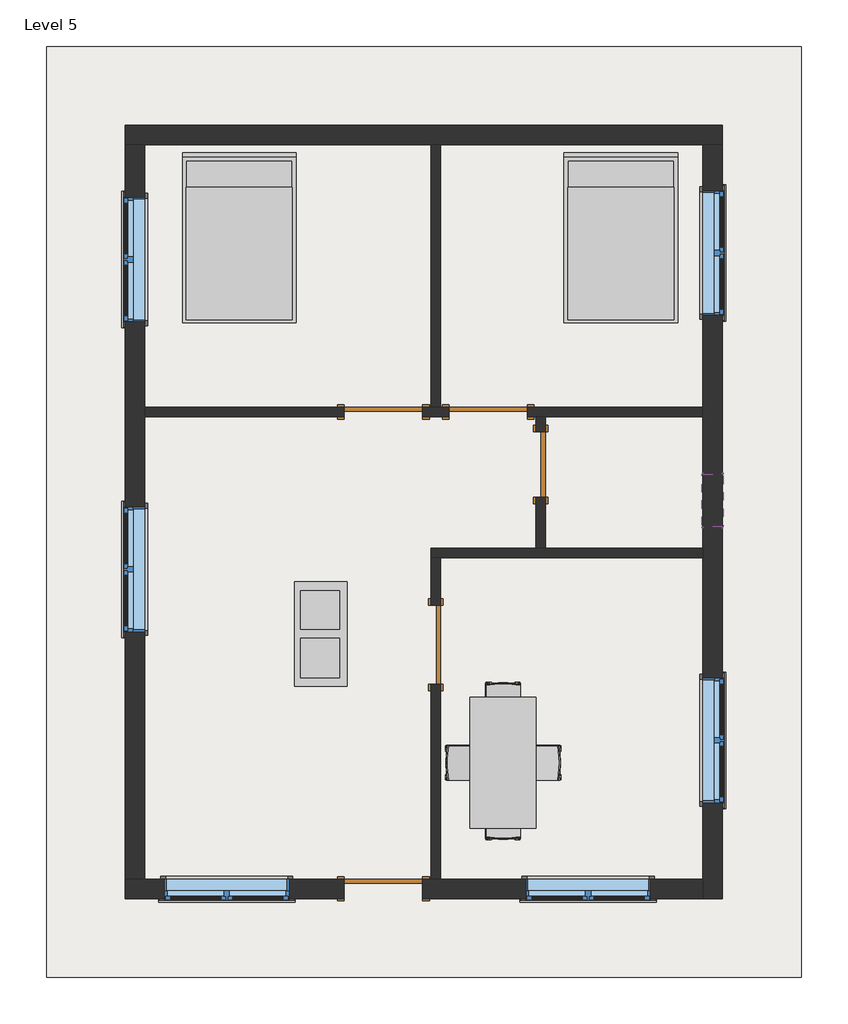
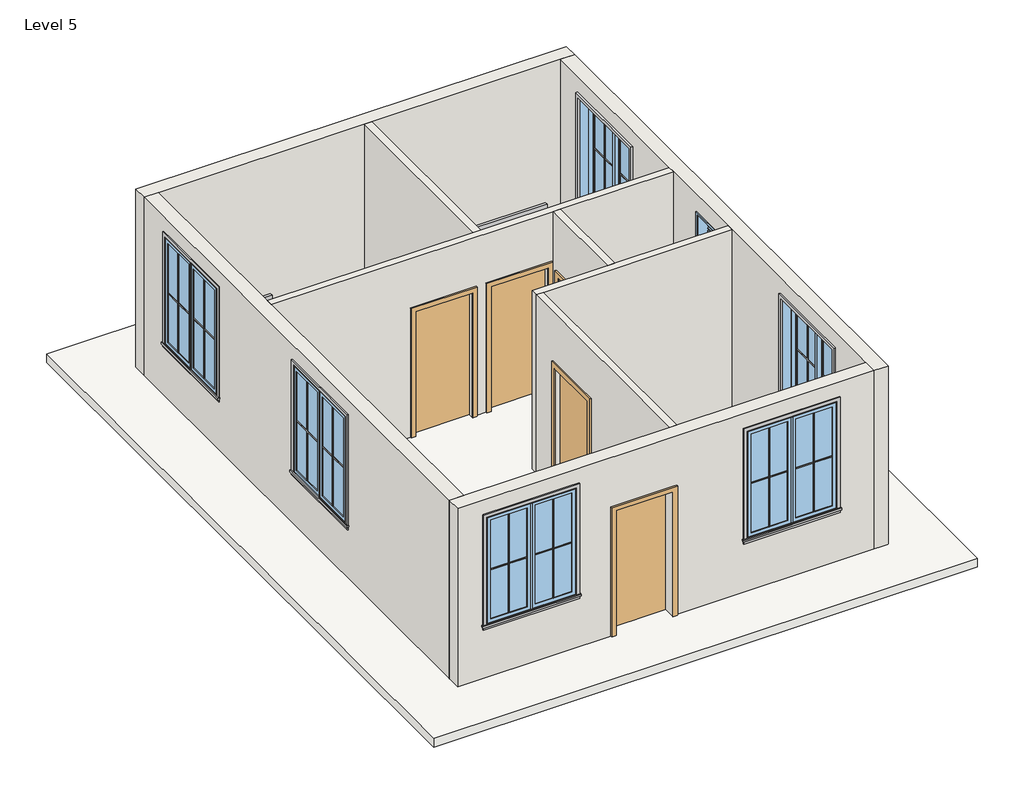
# One storey, incomplete: 25 proxies, 9 walls, 7 windows, 5 doors, 3 furniture elements, 1 roof.
"""IFC4 building model written with IfcOpenShell, lengths in millimetres."""

from ifc_helpers import new_model, si_unit, frame, origin, place, context, project, spatial, polyline, outline, extrude, faceted_brep, transform, mapped, element, save
from components import muntin_pattern_2x2_muntin_pattern_2x2_bff912c5, muntin_pattern_2x2_muntin_pattern_2x2_c2194282, trim_window_exterior_flat_with_sill_e04b3088, trim_window_interior_flat_picture_frame_2a7685fe, coffee_table_with_brass_mullions_11320_coffee_table_with_5962bef7, door_305aa2a5, door_e5f9f3c4, door_0ca8825f, door_f2b275c1, bed_17739_bed_17739_15c61121, dining_table_w_chairs_11374_0cdfc61b, window_9ac97e1a, window_f2d8fef0

model = new_model("IFC4")

# Units and contexts
model_context = context("Model", 3, world=origin())
ifc_project = project(units=[si_unit("LENGTHUNIT", "METRE", prefix="MILLI")], contexts=[model_context])

# Site, building, storey
site = spatial("IfcSite", under=ifc_project)
building = spatial("IfcBuilding", under=site)
storey = spatial("IfcBuildingStorey", under=building, Name="Level 5", Elevation=12649.2)

# Proxies
placement = place(None, origin())
muntin_pattern_2x2_muntin_pattern_2x2_shape = muntin_pattern_2x2_muntin_pattern_2x2_bff912c5(model_context)
element("IfcBuildingElementProxy", 1, Name="Muntin Pattern_2x2 : Muntin Pattern_2x2", ObjectType="Muntin Pattern_2x2 : Muntin Pattern_2x2", at=placement, inside=storey, context=model_context, shape_type="MappedRepresentation", body=[
    mapped(muntin_pattern_2x2_muntin_pattern_2x2_shape, transform((-4718.1437352, -1580.3188735, 13633.45), x_axis=(0.0, 1.0, 0.0), y_axis=(-1.0, 0.0, 0.0), z_axis=(0.0, 0.0, 1.0))),
])
element("IfcBuildingElementProxy", 2, Name="Muntin Pattern_2x2 : Muntin Pattern_2x2", ObjectType="Muntin Pattern_2x2 : Muntin Pattern_2x2", at=placement, inside=storey, context=model_context, shape_type="MappedRepresentation", body=[
    mapped(muntin_pattern_2x2_muntin_pattern_2x2_shape, transform((-3186.2062352, -5039.4813735, 13633.45), x_axis=(-1.0, 0.0, 0.0), y_axis=(0.0, -1.0, 0.0), z_axis=(0.0, 0.0, 1.0))),
])
element("IfcBuildingElementProxy", 3, Name="Muntin Pattern_2x2 : Muntin Pattern_2x2", ObjectType="Muntin Pattern_2x2 : Muntin Pattern_2x2", at=placement, inside=storey, context=model_context, shape_type="MappedRepresentation", body=[
    mapped(muntin_pattern_2x2_muntin_pattern_2x2_shape, transform((1017.4937648, -5039.4813735, 13633.45), x_axis=(-1.0, 0.0, 0.0), y_axis=(0.0, -1.0, 0.0), z_axis=(0.0, 0.0, 1.0))),
])
element("IfcBuildingElementProxy", 4, Name="Muntin Pattern_2x2 : Muntin Pattern_2x2", ObjectType="Muntin Pattern_2x2 : Muntin Pattern_2x2", at=placement, inside=storey, context=model_context, shape_type="MappedRepresentation", body=[
    mapped(muntin_pattern_2x2_muntin_pattern_2x2_shape, transform((2209.7062648, -2847.1438735, 13633.45), x_axis=(0.0, -1.0, 0.0), y_axis=(1.0, 0.0, 0.0), z_axis=(0.0, 0.0, 1.0))),
])
element("IfcBuildingElementProxy", 5, Name="Muntin Pattern_2x2 : Muntin Pattern_2x2", ObjectType="Muntin Pattern_2x2 : Muntin Pattern_2x2", at=placement, inside=storey, context=model_context, shape_type="MappedRepresentation", body=[
    mapped(muntin_pattern_2x2_muntin_pattern_2x2_shape, transform((2209.7062648, 2817.0561265, 13633.45), x_axis=(0.0, -1.0, 0.0), y_axis=(1.0, 0.0, 0.0), z_axis=(0.0, 0.0, 1.0))),
])
element("IfcBuildingElementProxy", 6, Name="Muntin Pattern_2x2 : Muntin Pattern_2x2", ObjectType="Muntin Pattern_2x2 : Muntin Pattern_2x2", at=placement, inside=storey, context=model_context, shape_type="MappedRepresentation", body=[
    mapped(muntin_pattern_2x2_muntin_pattern_2x2_shape, transform((-4718.1437352, 2020.1311265, 13633.45), x_axis=(0.0, 1.0, 0.0), y_axis=(-1.0, 0.0, 0.0), z_axis=(0.0, 0.0, 1.0))),
])
muntin_pattern_2x2_muntin_pattern_2x2_2_shape = muntin_pattern_2x2_muntin_pattern_2x2_c2194282(model_context)
element("IfcBuildingElementProxy", 7, Name="Muntin Pattern_2x2 : Muntin Pattern_2x2", ObjectType="Muntin Pattern_2x2 : Muntin Pattern_2x2", at=placement, inside=storey, context=model_context, shape_type="MappedRepresentation", body=[
    mapped(muntin_pattern_2x2_muntin_pattern_2x2_2_shape, transform((-4718.1437352, -859.5938735, 13633.45), x_axis=(0.0, -1.0, 0.0), y_axis=(1.0, 0.0, 0.0), z_axis=(0.0, 0.0, 1.0))),
])
element("IfcBuildingElementProxy", 8, Name="Muntin Pattern_2x2 : Muntin Pattern_2x2", ObjectType="Muntin Pattern_2x2 : Muntin Pattern_2x2", at=placement, inside=storey, context=model_context, shape_type="MappedRepresentation", body=[
    mapped(muntin_pattern_2x2_muntin_pattern_2x2_2_shape, transform((-3906.9312352, -5039.4813735, 13633.45), x_axis=(1.0, 0.0, 0.0), y_axis=(0.0, 1.0, 0.0), z_axis=(0.0, 0.0, 1.0))),
])
element("IfcBuildingElementProxy", 9, Name="Muntin Pattern_2x2 : Muntin Pattern_2x2", ObjectType="Muntin Pattern_2x2 : Muntin Pattern_2x2", at=placement, inside=storey, context=model_context, shape_type="MappedRepresentation", body=[
    mapped(muntin_pattern_2x2_muntin_pattern_2x2_2_shape, transform((296.7687648, -5039.4813735, 13633.45), x_axis=(1.0, 0.0, 0.0), y_axis=(0.0, 1.0, 0.0), z_axis=(0.0, 0.0, 1.0))),
])
element("IfcBuildingElementProxy", 10, Name="Muntin Pattern_2x2 : Muntin Pattern_2x2", ObjectType="Muntin Pattern_2x2 : Muntin Pattern_2x2", at=placement, inside=storey, context=model_context, shape_type="MappedRepresentation", body=[
    mapped(muntin_pattern_2x2_muntin_pattern_2x2_2_shape, transform((2209.7062648, -3567.8688735, 13633.45), x_axis=(0.0, 1.0, 0.0), y_axis=(-1.0, 0.0, 0.0), z_axis=(0.0, 0.0, 1.0))),
])
element("IfcBuildingElementProxy", 11, Name="Muntin Pattern_2x2 : Muntin Pattern_2x2", ObjectType="Muntin Pattern_2x2 : Muntin Pattern_2x2", at=placement, inside=storey, context=model_context, shape_type="MappedRepresentation", body=[
    mapped(muntin_pattern_2x2_muntin_pattern_2x2_2_shape, transform((2209.7062648, 2096.3311265, 13633.45), x_axis=(0.0, 1.0, 0.0), y_axis=(-1.0, 0.0, 0.0), z_axis=(0.0, 0.0, 1.0))),
])
element("IfcBuildingElementProxy", 12, Name="Muntin Pattern_2x2 : Muntin Pattern_2x2", ObjectType="Muntin Pattern_2x2 : Muntin Pattern_2x2", at=placement, inside=storey, context=model_context, shape_type="MappedRepresentation", body=[
    mapped(muntin_pattern_2x2_muntin_pattern_2x2_2_shape, transform((-4718.1437352, 2740.8561265, 13633.45), x_axis=(0.0, -1.0, 0.0), y_axis=(1.0, 0.0, 0.0), z_axis=(0.0, 0.0, 1.0))),
])
trim_window_exterior_flat_with_sill_shape = trim_window_exterior_flat_with_sill_e04b3088(model_context)
element("IfcBuildingElementProxy", 13, Name="Trim-Window-Exterior-Flat : with Sill", ObjectType="Trim-Window-Exterior-Flat : with Sill", at=placement, inside=storey, context=model_context, shape_type="MappedRepresentation", body=[
    mapped(trim_window_exterior_flat_with_sill_shape, transform((-4727.6687352, -1219.9563735, 15392.4), x_axis=(0.0, -1.0, 0.0), y_axis=(0.0, 0.0, 1.0), z_axis=(-1.0, 0.0, 0.0))),
])
element("IfcBuildingElementProxy", 14, Name="Trim-Window-Exterior-Flat : with Sill", ObjectType="Trim-Window-Exterior-Flat : with Sill", at=placement, inside=storey, context=model_context, shape_type="MappedRepresentation", body=[
    mapped(trim_window_exterior_flat_with_sill_shape, transform((-3546.5687352, -5049.0063735, 15392.4), x_axis=(1.0, 0.0, 0.0), y_axis=(0.0, 0.0, 1.0), z_axis=(0.0, -1.0, 0.0))),
])
element("IfcBuildingElementProxy", 15, Name="Trim-Window-Exterior-Flat : with Sill", ObjectType="Trim-Window-Exterior-Flat : with Sill", at=placement, inside=storey, context=model_context, shape_type="MappedRepresentation", body=[
    mapped(trim_window_exterior_flat_with_sill_shape, transform((657.1312648, -5049.0063735, 15392.4), x_axis=(1.0, 0.0, 0.0), y_axis=(0.0, 0.0, 1.0), z_axis=(0.0, -1.0, 0.0))),
])
element("IfcBuildingElementProxy", 16, Name="Trim-Window-Exterior-Flat : with Sill", ObjectType="Trim-Window-Exterior-Flat : with Sill", at=placement, inside=storey, context=model_context, shape_type="MappedRepresentation", body=[
    mapped(trim_window_exterior_flat_with_sill_shape, transform((2219.2312648, -3207.5063735, 15392.4), x_axis=(0.0, 1.0, 0.0), y_axis=(0.0, 0.0, 1.0), z_axis=(1.0, 0.0, 0.0))),
])
element("IfcBuildingElementProxy", 17, Name="Trim-Window-Exterior-Flat : with Sill", ObjectType="Trim-Window-Exterior-Flat : with Sill", at=placement, inside=storey, context=model_context, shape_type="MappedRepresentation", body=[
    mapped(trim_window_exterior_flat_with_sill_shape, transform((2219.2312648, 2456.6936265, 15392.4), x_axis=(0.0, 1.0, 0.0), y_axis=(0.0, 0.0, 1.0), z_axis=(1.0, 0.0, 0.0))),
])
element("IfcBuildingElementProxy", 18, Name="Trim-Window-Exterior-Flat : with Sill", ObjectType="Trim-Window-Exterior-Flat : with Sill", at=placement, inside=storey, context=model_context, shape_type="MappedRepresentation", body=[
    mapped(trim_window_exterior_flat_with_sill_shape, transform((-4727.6687352, 2380.4936265, 15392.4), x_axis=(0.0, -1.0, 0.0), y_axis=(0.0, 0.0, 1.0), z_axis=(-1.0, 0.0, 0.0))),
])
trim_window_interior_flat_picture_frame_shape = trim_window_interior_flat_picture_frame_2a7685fe(model_context)
element("IfcBuildingElementProxy", 19, Name="Trim-Window-Interior-Flat : Picture Frame", ObjectType="Trim-Window-Interior-Flat : Picture Frame", at=placement, inside=storey, context=model_context, shape_type="MappedRepresentation", body=[
    mapped(trim_window_interior_flat_picture_frame_shape, transform((-4499.0687352, -1219.9563735, 15392.4), x_axis=(0.0, 1.0, 0.0), y_axis=(0.0, 0.0, 1.0), z_axis=(1.0, 0.0, 0.0))),
])
element("IfcBuildingElementProxy", 20, Name="Trim-Window-Interior-Flat : Picture Frame", ObjectType="Trim-Window-Interior-Flat : Picture Frame", at=placement, inside=storey, context=model_context, shape_type="MappedRepresentation", body=[
    mapped(trim_window_interior_flat_picture_frame_shape, transform((-3546.5687352, -4820.4063735, 15392.4), x_axis=(-1.0, 0.0, 0.0), y_axis=(0.0, 0.0, 1.0), z_axis=(0.0, 1.0, 0.0))),
])
element("IfcBuildingElementProxy", 21, Name="Trim-Window-Interior-Flat : Picture Frame", ObjectType="Trim-Window-Interior-Flat : Picture Frame", at=placement, inside=storey, context=model_context, shape_type="MappedRepresentation", body=[
    mapped(trim_window_interior_flat_picture_frame_shape, transform((657.1312648, -4820.4063735, 15392.4), x_axis=(-1.0, 0.0, 0.0), y_axis=(0.0, 0.0, 1.0), z_axis=(0.0, 1.0, 0.0))),
])
element("IfcBuildingElementProxy", 22, Name="Trim-Window-Interior-Flat : Picture Frame", ObjectType="Trim-Window-Interior-Flat : Picture Frame", at=placement, inside=storey, context=model_context, shape_type="MappedRepresentation", body=[
    mapped(trim_window_interior_flat_picture_frame_shape, transform((1990.6312648, -3207.5063735, 15392.4), x_axis=(0.0, -1.0, 0.0), y_axis=(0.0, 0.0, 1.0), z_axis=(-1.0, 0.0, 0.0))),
])
element("IfcBuildingElementProxy", 23, Name="Trim-Window-Interior-Flat : Picture Frame", ObjectType="Trim-Window-Interior-Flat : Picture Frame", at=placement, inside=storey, context=model_context, shape_type="MappedRepresentation", body=[
    mapped(trim_window_interior_flat_picture_frame_shape, transform((1990.6312648, 2456.6936265, 15392.4), x_axis=(0.0, -1.0, 0.0), y_axis=(0.0, 0.0, 1.0), z_axis=(-1.0, 0.0, 0.0))),
])
element("IfcBuildingElementProxy", 24, Name="Trim-Window-Interior-Flat : Picture Frame", ObjectType="Trim-Window-Interior-Flat : Picture Frame", at=placement, inside=storey, context=model_context, shape_type="MappedRepresentation", body=[
    mapped(trim_window_interior_flat_picture_frame_shape, transform((-4499.0687352, 2380.4936265, 15392.4), x_axis=(0.0, 1.0, 0.0), y_axis=(0.0, 0.0, 1.0), z_axis=(1.0, 0.0, 0.0))),
])
coffee_table_with_brass_mullions_11320_coffee_table_with_shape = coffee_table_with_brass_mullions_11320_coffee_table_with_5962bef7(model_context)
element("IfcBuildingElementProxy", 25, Name="coffee_table_with_brass_mullions_11320 : coffee_table_with_brass_mullions_11320", ObjectType="coffee_table_with_brass_mullions_11320 : coffee_table_with_brass_mullions_11320", at=placement, inside=storey, context=model_context, shape_type="MappedRepresentation", body=[
    mapped(coffee_table_with_brass_mullions_11320_coffee_table_with_shape, transform((-2022.5687352, -1334.2563735, 12649.2), x_axis=(0.0, 1.0, 0.0), y_axis=(-1.0, 0.0, 0.0), z_axis=(0.0, 0.0, 1.0))),
])

# Doors
door_shape = door_305aa2a5(model_context)
element("IfcDoor", 26, ObjectType="Single-Flush : 36\" x 84\"", at=placement, inside=storey, context=model_context, shape_type="MappedRepresentation", body=[
    mapped(door_shape, transform((-1114.5187352, -2096.2563735, 12649.2), x_axis=(0.0, 1.0, 0.0), y_axis=(-1.0, 0.0, 0.0), z_axis=(0.0, 0.0, 1.0))),
])
element("IfcDoor", 27, ObjectType="Single-Flush : 36\" x 84\"", at=placement, inside=storey, context=model_context, shape_type="MappedRepresentation", body=[
    mapped(door_shape, transform((-1724.1187352, 608.8436265, 12649.2), x_axis=(-1.0, 0.0, 0.0), y_axis=(0.0, -1.0, 0.0), z_axis=(0.0, 0.0, 1.0))),
])
door_2_shape = door_e5f9f3c4(model_context)
element("IfcDoor", 28, ObjectType="Single-Flush : 36\" x 84\"", at=placement, inside=storey, context=model_context, shape_type="MappedRepresentation", body=[
    mapped(door_2_shape, transform((-504.9187352, 608.8436265, 12649.2), x_axis=(1.0, 0.0, 0.0), y_axis=(0.0, 1.0, 0.0), z_axis=(0.0, 0.0, 1.0))),
])
door_3_shape = door_0ca8825f(model_context)
element("IfcDoor", 29, ObjectType="Single-Flush : 36\" x 84\"", at=placement, inside=storey, context=model_context, shape_type="MappedRepresentation", body=[
    mapped(door_3_shape, transform((-1724.1187352, -4934.7063735, 12649.2), x_axis=(1.0, 0.0, 0.0), y_axis=(0.0, 1.0, 0.0), z_axis=(0.0, 0.0, 1.0))),
])
door_4_shape = door_f2b275c1(model_context)
element("IfcDoor", 30, ObjectType="Single-Flush : DOOR 2'6\"", at=placement, inside=storey, context=model_context, shape_type="MappedRepresentation", body=[
    mapped(door_4_shape, transform((104.6812648, -0.7563735, 12649.2), x_axis=(0.0, 1.0, 0.0), y_axis=(-1.0, 0.0, 0.0), z_axis=(0.0, 0.0, 1.0))),
])

# Furniture
bed_17739_bed_17739_shape = bed_17739_bed_17739_15c61121(model_context)
element("IfcFurniture", 31, ObjectType="Bed_17739 : Bed_17739", at=placement, inside=storey, context=model_context, shape_type="MappedRepresentation", body=[
    mapped(bed_17739_bed_17739_shape, transform((-3400.5187352, 2609.0936265, 12649.2), x_axis=(1.0, 0.0, 0.0), y_axis=(0.0, 1.0, 0.0), z_axis=(0.0, 0.0, 1.0))),
])
element("IfcFurniture", 32, ObjectType="Bed_17739 : Bed_17739", at=placement, inside=storey, context=model_context, shape_type="MappedRepresentation", body=[
    mapped(bed_17739_bed_17739_shape, transform((1038.1312648, 2609.0936265, 12649.2), x_axis=(1.0, 0.0, 0.0), y_axis=(0.0, 1.0, 0.0), z_axis=(0.0, 0.0, 1.0))),
])
dining_table_w_chairs_11374_shape = dining_table_w_chairs_11374_0cdfc61b(model_context)
element("IfcFurniture", 33, ObjectType="Dining_Table_w_Chairs_11374", at=placement, inside=storey, context=model_context, shape_type="MappedRepresentation", body=[
    mapped(dining_table_w_chairs_11374_shape, transform((-238.2576574, -3486.1221401, 12649.2), x_axis=(0.0, 1.0, 0.0), y_axis=(-1.0, 0.0, 0.0), z_axis=(0.0, 0.0, 1.0))),
])

# Roof
element("IfcRoof", 34, ObjectType="ROOF 6\"", at=placement, inside=storey, context=model_context, shape_type="SweptSolid", body=[
    extrude(outline(polyline([(-5642.0687352, 4856.9936265), (3133.6312648, 4856.9936265), (3133.6312648, -5963.4063735), (-5642.0687352, -5963.4063735), (-5642.0687352, 4856.9936265)])), frame((0.0, 0.0, 12496.8), z_axis=(0.0, 0.0, 1.0), x_axis=(1.0, 0.0, 0.0)), (0.0, 0.0, 1.0), 152.4),
])

# Walls
element("IfcWall", 35, ObjectType="WALL 4.5\"", at=placement, inside=storey, context=model_context, shape_type="Brep", body=[
    faceted_brep([(-4499.0687352, 551.6936265, 12649.2), (-2181.3187352, 551.6936265, 12649.2), (-2181.3187352, 551.6936265, 14782.8), (-1266.9187352, 551.6936265, 14782.8), (-1266.9187352, 551.6936265, 12649.2), (-962.1187352, 551.6936265, 12649.2), (-962.1187352, 551.6936265, 14782.8), (-47.7187352, 551.6936265, 14782.8), (-47.7187352, 551.6936265, 12649.2), (47.5312648, 551.6936265, 12649.2), (161.8312648, 551.6936265, 12649.2), (1990.6312648, 551.6936265, 12649.2), (1990.6312648, 551.6936265, 15697.2), (161.8312648, 551.6936265, 15697.2), (47.5312648, 551.6936265, 15697.2), (-4499.0687352, 551.6936265, 15697.2), (-2181.3187352, 665.9936265, 14782.8), (-2181.3187352, 665.9936265, 12649.2), (-4499.0687352, 665.9936265, 12649.2), (-4499.0687352, 665.9936265, 15697.2), (-1171.6687352, 665.9936265, 15697.2), (-1057.3687352, 665.9936265, 15697.2), (1990.6312648, 665.9936265, 15697.2), (1990.6312648, 665.9936265, 12649.2), (-47.7187352, 665.9936265, 12649.2), (-47.7187352, 665.9936265, 14782.8), (-962.1187352, 665.9936265, 14782.8), (-962.1187352, 665.9936265, 12649.2), (-1057.3687352, 665.9936265, 12649.2), (-1171.6687352, 665.9936265, 12649.2), (-1266.9187352, 665.9936265, 12649.2), (-1266.9187352, 665.9936265, 14782.8)], [[[0, 1, 2, 3, 4, 5, 6, 7, 8, 9, 10, 11, 12, 13, 14, 15]], [[16, 17, 18, 19, 20, 21, 22, 23, 24, 25, 26, 27, 28, 29, 30, 31]], [[11, 10, 9, 8, 24, 23]], [[18, 17, 1, 0]], [[30, 29, 28, 27, 5, 4]], [[12, 11, 23, 22]], [[0, 15, 19, 18]], [[25, 24, 8, 7]], [[26, 25, 7, 6]], [[27, 26, 6, 5]], [[2, 1, 17, 16]], [[3, 2, 16, 31]], [[4, 3, 31, 30]], [[15, 14, 13, 12, 22, 21, 20, 19]]]),
])
element("IfcWall", 36, ObjectType="WALL 4.5\"", at=placement, inside=storey, context=model_context, shape_type="SweptSolid", body=[
    extrude(outline(polyline([(-1057.3687352, 3713.9936265), (-1057.3687352, 665.9936265), (-1171.6687352, 665.9936265), (-1171.6687352, 3713.9936265), (-1057.3687352, 3713.9936265)])), frame((0.0, 0.0, 12649.2), z_axis=(0.0, 0.0, 1.0), x_axis=(1.0, 0.0, 0.0)), (0.0, 0.0, 1.0), 3048.0),
])
element("IfcWall", 37, ObjectType="WALL 4.5\"", at=placement, inside=storey, context=model_context, shape_type="Brep", body=[
    faceted_brep([(1990.6312648, -972.3063735, 12649.2), (161.8312648, -972.3063735, 12649.2), (47.5312648, -972.3063735, 12649.2), (-1171.6687352, -972.3063735, 12649.2), (-1171.6687352, -972.3063735, 15697.2), (47.5312648, -972.3063735, 15697.2), (161.8312648, -972.3063735, 15697.2), (1990.6312648, -972.3063735, 15697.2), (1990.6312648, -1086.6063735, 12649.2), (1990.6312648, -1086.6063735, 15697.2), (-1057.3687352, -1086.6063735, 15697.2), (-1171.6687352, -1086.6063735, 15697.2), (-1171.6687352, -1086.6063735, 12649.2), (-1057.3687352, -1086.6063735, 12649.2)], [[[0, 1, 2, 3, 4, 5, 6, 7]], [[8, 9, 10, 11, 12, 13]], [[3, 2, 1, 0, 8, 13, 12]], [[0, 7, 9, 8]], [[4, 3, 12, 11]], [[7, 6, 5, 4, 11, 10, 9]]]),
])
element("IfcWall", 38, ObjectType="WALL 4.5\"", at=placement, inside=storey, context=model_context, shape_type="SweptSolid", body=[
    extrude(outline(polyline([(-1086.6063735, 12649.2), (-1639.0563735, 12649.2), (-1639.0563735, 14782.8), (-2553.4563735, 14782.8), (-2553.4563735, 12649.2), (-4820.4063735, 12649.2), (-4820.4063735, 15697.2), (-1086.6063735, 15697.2), (-1086.6063735, 12649.2)])), frame((-1171.6687352, 0.0, 0.0), z_axis=(1.0, 0.0, 0.0), x_axis=(0.0, 1.0, 0.0)), (0.0, 0.0, 1.0), 114.3),
])
element("IfcWall", 39, ObjectType="WALL 4.5\"", at=placement, inside=storey, context=model_context, shape_type="SweptSolid", body=[
    extrude(outline(polyline([(551.6936265, 12649.2), (380.2436265, 12649.2), (380.2436265, 14681.2), (-381.7563735, 14681.2), (-381.7563735, 12649.2), (-972.3063735, 12649.2), (-972.3063735, 15697.2), (551.6936265, 15697.2), (551.6936265, 12649.2)])), frame((47.5312648, 0.0, 0.0), z_axis=(1.0, 0.0, 0.0), x_axis=(0.0, 1.0, 0.0)), (0.0, 0.0, 1.0), 114.3),
])
element("IfcWall", 40, ObjectType="WALL 9\"", at=placement, inside=storey, context=model_context, shape_type="Brep", body=[
    faceted_brep([(-4727.6687352, 3713.9936265, 12649.2), (-4499.0687352, 3713.9936265, 12649.2), (-1171.6687352, 3713.9936265, 12649.2), (-1057.3687352, 3713.9936265, 12649.2), (1990.6312648, 3713.9936265, 12649.2), (2219.2312648, 3713.9936265, 12649.2), (2219.2312648, 3713.9936265, 15697.2), (1990.6312648, 3713.9936265, 15697.2), (-1057.3687352, 3713.9936265, 15697.2), (-1171.6687352, 3713.9936265, 15697.2), (-4499.0687352, 3713.9936265, 15697.2), (-4727.6687352, 3713.9936265, 15697.2), (-4727.6687352, 3942.5936265, 12649.2), (-4727.6687352, 3942.5936265, 15697.2), (2219.2312648, 3942.5936265, 15697.2), (2219.2312648, 3942.5936265, 12649.2)], [[[0, 1, 2, 3, 4, 5, 6, 7, 8, 9, 10, 11]], [[12, 13, 14, 15]], [[5, 4, 3, 2, 1, 0, 12, 15]], [[6, 5, 15, 14]], [[0, 11, 13, 12]], [[11, 10, 9, 8, 7, 6, 14, 13]]]),
])
element("IfcWall", 41, ObjectType="WALL 9\"", at=placement, inside=storey, context=model_context, shape_type="Brep", body=[
    faceted_brep([(1990.6312648, 3713.9936265, 12649.2), (1990.6312648, 665.9936265, 12649.2), (1990.6312648, 551.6936265, 12649.2), (1990.6312648, -972.3063735, 12649.2), (1990.6312648, -1086.6063735, 12649.2), (1990.6312648, -4820.4063735, 12649.2), (1990.6312648, -5049.0063735, 12649.2), (1990.6312648, -5049.0063735, 15697.2), (1990.6312648, -4820.4063735, 15697.2), (1990.6312648, -1086.6063735, 15697.2), (1990.6312648, -972.3063735, 15697.2), (1990.6312648, 551.6936265, 15697.2), (1990.6312648, 665.9936265, 15697.2), (1990.6312648, 3713.9936265, 15697.2), (1990.6312648, -3931.4063735, 15392.4), (1990.6312648, -3931.4063735, 13563.6), (1990.6312648, -2483.6063735, 13563.6), (1990.6312648, -2483.6063735, 15392.4), (1990.6312648, 1732.7936265, 15392.4), (1990.6312648, 1732.7936265, 13563.6), (1990.6312648, 3180.5936265, 13563.6), (1990.6312648, 3180.5936265, 15392.4), (1990.6312648, -115.0563735, 15392.4), (1990.6312648, -724.6563735, 15392.4), (1990.6312648, -724.6563735, 14782.8), (1990.6312648, -115.0563735, 14782.8), (2219.2312648, 3713.9936265, 12649.2), (2219.2312648, 3713.9936265, 15697.2), (2219.2312648, -5049.0063735, 15697.2), (2219.2312648, -5049.0063735, 12649.2), (2219.2312648, -3931.4063735, 15392.4), (2219.2312648, -2483.6063735, 15392.4), (2219.2312648, -2483.6063735, 13563.6), (2219.2312648, -3931.4063735, 13563.6), (2219.2312648, 1732.7936265, 15392.4), (2219.2312648, 3180.5936265, 15392.4), (2219.2312648, 3180.5936265, 13563.6), (2219.2312648, 1732.7936265, 13563.6), (2219.2312648, -115.0563735, 15392.4), (2219.2312648, -115.0563735, 14782.8), (2219.2312648, -724.6563735, 14782.8), (2219.2312648, -724.6563735, 15392.4)], [[[0, 1, 2, 3, 4, 5, 6, 7, 8, 9, 10, 11, 12, 13], [14, 15, 16, 17], [18, 19, 20, 21], [22, 23, 24, 25]], [[26, 27, 28, 29], [30, 31, 32, 33], [34, 35, 36, 37], [38, 39, 40, 41]], [[6, 5, 4, 3, 2, 1, 0, 26, 29]], [[0, 13, 27, 26]], [[7, 6, 29, 28]], [[15, 14, 30, 33]], [[16, 15, 33, 32]], [[17, 16, 32, 31]], [[14, 17, 31, 30]], [[19, 18, 34, 37]], [[20, 19, 37, 36]], [[21, 20, 36, 35]], [[18, 21, 35, 34]], [[39, 38, 22, 25]], [[40, 39, 25, 24]], [[41, 40, 24, 23]], [[38, 41, 23, 22]], [[13, 12, 11, 10, 9, 8, 7, 28, 27]]]),
])
element("IfcWall", 42, ObjectType="WALL 9\"", at=placement, inside=storey, context=model_context, shape_type="Brep", body=[
    faceted_brep([(1990.6312648, -4820.4063735, 12649.2), (-1057.3687352, -4820.4063735, 12649.2), (-1171.6687352, -4820.4063735, 12649.2), (-1266.9187352, -4820.4063735, 12649.2), (-1266.9187352, -4820.4063735, 14782.8), (-2181.3187352, -4820.4063735, 14782.8), (-2181.3187352, -4820.4063735, 12649.2), (-4499.0687352, -4820.4063735, 12649.2), (-4727.6687352, -4820.4063735, 12649.2), (-4727.6687352, -4820.4063735, 15697.2), (-4499.0687352, -4820.4063735, 15697.2), (-1171.6687352, -4820.4063735, 15697.2), (-1057.3687352, -4820.4063735, 15697.2), (1990.6312648, -4820.4063735, 15697.2), (-4270.4687352, -4820.4063735, 15392.4), (-4270.4687352, -4820.4063735, 13563.6), (-2822.6687352, -4820.4063735, 13563.6), (-2822.6687352, -4820.4063735, 15392.4), (-66.7687352, -4820.4063735, 15392.4), (-66.7687352, -4820.4063735, 13563.6), (1381.0312648, -4820.4063735, 13563.6), (1381.0312648, -4820.4063735, 15392.4), (-1266.9187352, -5049.0063735, 14782.8), (-1266.9187352, -5049.0063735, 12649.2), (1990.6312648, -5049.0063735, 12649.2), (1990.6312648, -5049.0063735, 15697.2), (-4727.6687352, -5049.0063735, 15697.2), (-4727.6687352, -5049.0063735, 12649.2), (-2181.3187352, -5049.0063735, 12649.2), (-2181.3187352, -5049.0063735, 14782.8), (-4270.4687352, -5049.0063735, 15392.4), (-2822.6687352, -5049.0063735, 15392.4), (-2822.6687352, -5049.0063735, 13563.6), (-4270.4687352, -5049.0063735, 13563.6), (-66.7687352, -5049.0063735, 15392.4), (1381.0312648, -5049.0063735, 15392.4), (1381.0312648, -5049.0063735, 13563.6), (-66.7687352, -5049.0063735, 13563.6)], [[[0, 1, 2, 3, 4, 5, 6, 7, 8, 9, 10, 11, 12, 13], [14, 15, 16, 17], [18, 19, 20, 21]], [[22, 23, 24, 25, 26, 27, 28, 29], [30, 31, 32, 33], [34, 35, 36, 37]], [[28, 27, 8, 7, 6]], [[24, 23, 3, 2, 1, 0]], [[0, 13, 25, 24]], [[9, 8, 27, 26]], [[15, 14, 30, 33]], [[16, 15, 33, 32]], [[17, 16, 32, 31]], [[14, 17, 31, 30]], [[19, 18, 34, 37]], [[20, 19, 37, 36]], [[21, 20, 36, 35]], [[18, 21, 35, 34]], [[4, 3, 23, 22]], [[5, 4, 22, 29]], [[6, 5, 29, 28]], [[13, 12, 11, 10, 9, 26, 25]]]),
])
element("IfcWall", 43, ObjectType="WALL 9\"", at=placement, inside=storey, context=model_context, shape_type="Brep", body=[
    faceted_brep([(-4499.0687352, -4820.4063735, 12649.2), (-4499.0687352, 551.6936265, 12649.2), (-4499.0687352, 665.9936265, 12649.2), (-4499.0687352, 3713.9936265, 12649.2), (-4499.0687352, 3713.9936265, 15697.2), (-4499.0687352, 665.9936265, 15697.2), (-4499.0687352, 551.6936265, 15697.2), (-4499.0687352, -4820.4063735, 15697.2), (-4499.0687352, -496.0563735, 15392.4), (-4499.0687352, -496.0563735, 13563.6), (-4499.0687352, -1943.8563735, 13563.6), (-4499.0687352, -1943.8563735, 15392.4), (-4499.0687352, 3104.3936265, 15392.4), (-4499.0687352, 3104.3936265, 13563.6), (-4499.0687352, 1656.5936265, 13563.6), (-4499.0687352, 1656.5936265, 15392.4), (-4727.6687352, -4820.4063735, 12649.2), (-4727.6687352, -4820.4063735, 15697.2), (-4727.6687352, 3713.9936265, 15697.2), (-4727.6687352, 3713.9936265, 12649.2), (-4727.6687352, -496.0563735, 15392.4), (-4727.6687352, -1943.8563735, 15392.4), (-4727.6687352, -1943.8563735, 13563.6), (-4727.6687352, -496.0563735, 13563.6), (-4727.6687352, 3104.3936265, 15392.4), (-4727.6687352, 1656.5936265, 15392.4), (-4727.6687352, 1656.5936265, 13563.6), (-4727.6687352, 3104.3936265, 13563.6)], [[[0, 1, 2, 3, 4, 5, 6, 7], [8, 9, 10, 11], [12, 13, 14, 15]], [[16, 17, 18, 19], [20, 21, 22, 23], [24, 25, 26, 27]], [[3, 2, 1, 0, 16, 19]], [[4, 3, 19, 18]], [[0, 7, 17, 16]], [[9, 8, 20, 23]], [[10, 9, 23, 22]], [[11, 10, 22, 21]], [[8, 11, 21, 20]], [[13, 12, 24, 27]], [[14, 13, 27, 26]], [[15, 14, 26, 25]], [[12, 15, 25, 24]], [[7, 6, 5, 4, 18, 17]]]),
])

# Windows
window_shape = window_9ac97e1a(model_context)
element("IfcWindow", 44, ObjectType="Window-Casement-Double : 57\" x 72\"", at=placement, inside=storey, context=model_context, shape_type="MappedRepresentation", body=[
    mapped(window_shape, transform((-4613.3687352, -1219.9563735, 12649.2), x_axis=(0.0, 1.0, 0.0), y_axis=(-1.0, 0.0, 0.0), z_axis=(0.0, 0.0, 1.0))),
])
element("IfcWindow", 45, ObjectType="Window-Casement-Double : 57\" x 72\"", at=placement, inside=storey, context=model_context, shape_type="MappedRepresentation", body=[
    mapped(window_shape, transform((-3546.5687352, -4934.7063735, 12649.2), x_axis=(-1.0, 0.0, 0.0), y_axis=(0.0, -1.0, 0.0), z_axis=(0.0, 0.0, 1.0))),
])
element("IfcWindow", 46, ObjectType="Window-Casement-Double : 57\" x 72\"", at=placement, inside=storey, context=model_context, shape_type="MappedRepresentation", body=[
    mapped(window_shape, transform((657.1312648, -4934.7063735, 12649.2), x_axis=(-1.0, 0.0, 0.0), y_axis=(0.0, -1.0, 0.0), z_axis=(0.0, 0.0, 1.0))),
])
element("IfcWindow", 47, ObjectType="Window-Casement-Double : 57\" x 72\"", at=placement, inside=storey, context=model_context, shape_type="MappedRepresentation", body=[
    mapped(window_shape, transform((2104.9312648, -3207.5063735, 12649.2), x_axis=(0.0, -1.0, 0.0), y_axis=(1.0, 0.0, 0.0), z_axis=(0.0, 0.0, 1.0))),
])
element("IfcWindow", 48, ObjectType="Window-Casement-Double : 57\" x 72\"", at=placement, inside=storey, context=model_context, shape_type="MappedRepresentation", body=[
    mapped(window_shape, transform((2104.9312648, 2456.6936265, 12649.2), x_axis=(0.0, -1.0, 0.0), y_axis=(1.0, 0.0, 0.0), z_axis=(0.0, 0.0, 1.0))),
])
element("IfcWindow", 49, ObjectType="Window-Casement-Double : 57\" x 72\"", at=placement, inside=storey, context=model_context, shape_type="MappedRepresentation", body=[
    mapped(window_shape, transform((-4613.3687352, 2380.4936265, 12649.2), x_axis=(0.0, 1.0, 0.0), y_axis=(-1.0, 0.0, 0.0), z_axis=(0.0, 0.0, 1.0))),
])
window_2_shape = window_f2d8fef0(model_context)
element("IfcWindow", 50, ObjectType="Window-Louvers : 24\" x 24\"", at=placement, inside=storey, context=model_context, shape_type="MappedRepresentation", body=[
    mapped(window_2_shape, transform((2111.2812648, -419.8563735, 13868.4), x_axis=(0.0, -1.0, 0.0), y_axis=(1.0, 0.0, 0.0), z_axis=(0.0, 0.0, 1.0))),
])

save(model, "model.ifc")

# Revit data of these elements
# Type "Muntin Pattern_2x2 : Muntin Pattern_2x2"
#   Width [instance default] = 4' - 0"
#   Thickness = 0' - 0 1/2"
#   Height [instance default] = 4' - 0"
#   Distance = 0' - 0 3/4"
#   Interior Material [instance default] = none
#   Exterior Material [instance default] = none
#   Default Elevation = 0
# Type "Trim-Window-Exterior-Flat : with Sill"
#   Trim Width = 0' - 2 1/4"
#   Trim Thickness_Picture Frame = 0' - 1 1/4"
#   Trim Thickness_with Sill = 0' - 0 3/4"
#   Sill Thickness = 0' - 1 1/4"
#   Opening Width [instance default] = 2' - 0"
#   Opening Height [instance default] = 3' - 0"
#   Default Elevation = 4' - 0"
#   Sill = yes
#   Picture Frame = no
#   Trim Material [instance default] = none
# Type "Trim-Window-Interior-Flat : Picture Frame"
#   Trim Thickness_Picture Frame = 0' - 1 1/4"
#   Trim Width = 0' - 2 1/4"
#   Trim Thickness_with Sill = 0' - 0 3/4"
#   Sill Thickness = 0' - 1 1/4"
#   Opening Width [instance default] = 2' - 0"
#   Opening Height [instance default] = 3' - 0"
#   Default Elevation = 4' - 0"
#   Sill = no
#   Picture Frame = yes
#   Trim Material [instance default] = none
# Type "coffee_table_with_brass_mullions_11320 : coffee_table_with_brass_mullions_11320"
#   Default Elevation = 0
# Type "Single-Flush : 36\" x 84\""
#   Type Mark = "1"
#   Construction Type Id = "MDOOR"
#   Assembly Code = "C1020"
#   Analytic Construction = "Metal"
#   Thickness = 0' - 2"
#   Heat Transfer Coefficient (U) = 0.651978 BTU/(h·ft²·°F)
#   Height = 7' - 0"
#   Trim Projection Ext = 0' - 1"
#   Trim Projection Int = 0' - 1"
#   Trim Width = 0' - 3"
#   Width = 3' - 0"
#   Define Thermal Properties by = 1
#   Define Thermal Properties by = 1
#   Door Material = Door - Panel
#   Frame Material = Door - Frame
#   Visual Light Transmittance = 0
#   Solar Heat Gain Coefficient = 0
#   Function = (empty or 0)
#   Wall Closure = (empty or 0)
# Type "Single-Flush : DOOR 2'6\""
#   Type Mark = "8"
#   Construction Type Id = "MDOOR"
#   Assembly Code = "C1020"
#   Analytic Construction = "Metal"
#   Thickness = 0' - 2"
#   Heat Transfer Coefficient (U) = 0.651978 BTU/(h·ft²·°F)
#   Height = 6' - 8"
#   Trim Projection Ext = 0' - 1"
#   Trim Projection Int = 0' - 1"
#   Trim Width = 0' - 3"
#   Width = 2' - 6"
#   Define Thermal Properties by = 1
#   Door Material = Door - Panel
#   Frame Material = Door - Frame
#   Visual Light Transmittance = 0
#   Solar Heat Gain Coefficient = 0
#   Function = (empty or 0)
#   Wall Closure = (empty or 0)
# Type "Bed_17739 : Bed_17739"
#   Default Elevation = 0
# Type "Dining_Table_w_Chairs_11374"
#   Default Elevation = 0
#   Assembly Code = ""
# Type "ROOF 6\""
#   Assembly Code = "B1020"
#   Layers, outside or top first: 0' - 6" no material (function 1)
# Type "WALL 4.5\""
#   Assembly Code = "B2010"
#   Layers, outside or top first: 0' - 4 1/2" no material (function 1)
# Type "WALL 9\""
#   Assembly Code = "B2010"
#   Layers, outside or top first: 0' - 9" no material (function 1)
# Type "Window-Casement-Double : 57\" x 72\""
#   Type Mark = "17"
#   Fire Rating = "0.5h"
#   Assembly Code = "B2020100"
#   Analytic Construction = "Double glazing - domestic"
#   Frame Extension [instance default] = 0' - 0 1/4"
#   Window Inset [instance default] = 0' - 0"
#   Wall Thickness [instance default] = 0' - 6"
#   Interior Wall Closure [instance default] = 0' - 2 1/4"
#   Half Width = 2' - 4 1/2"
#   Visual Light Transmittance = 0.81
#   Thermal Resistance (R) = 1.8146 (h·ft²·°F)/BTU
#   Solar Heat Gain Coefficient = 0.76
#   Rough Width = 4' - 9 1/2"
#   Rough Height = 6' - 0 1/2"
#   Height = 6' - 0"
#   Heat Transfer Coefficient (U) = 0.5511 BTU/(h·ft²·°F)
#   Exterior Wall Closure [instance default] = 0' - 1 1/4"
#   Extension Jamb [instance default] = 0' - 2 1/4"
#   Default Sill Height = 3' - 0"
#   Width = 4' - 9"
#   Define Thermal Properties by = 0
#   Muntin Visibility = yes
#   Interior Trim Visibility [instance default] = yes
#   Exterior Trim Visibility [instance default] = yes
#   Extension Jamb Visibility [instance default] = yes
#   Interior Trim Material = Wood - Stained
#   Muntin Pattern = Muntin Pattern_2x2 : Muntin Pattern_2x2
#   Interior Trim = Trim-Window-Interior-Flat : Picture Frame
#   Interior Frame Material = Wood - Stained
#   Glass Panel Material = Glass
#   Exterior Trim Material = Clad - White
#   Exterior Trim = Trim-Window-Exterior-Flat : with Sill
#   Exterior Frame Material = Clad - White
#   Wall Closure = (empty or 0)
# Type "Window-Louvers : 24\" x 24\""
#   Type Mark = "18"
#   Construction Type Id = "GSP4R"
#   Assembly Code = "B20"
#   Analytic Construction = "1/8 in Pilkington single glazing"
#   Visual Light Transmittance = 0.9
#   Thermal Resistance (R) = 1.53941 (h·ft²·°F)/BTU
#   Solar Heat Gain Coefficient = 0.78
#   Max Height = 1' - 11.74264"
#   Height = 2' - 0"
#   Heat Transfer Coefficient (U) = 0.6496 BTU/(h·ft²·°F)
#   Blade Width [instance default] = 1' - 10 1/2"
#   Blade Vertical Thickness = 0' - 0.35355"
#   Blade Thickness = 0' - 0 1/4"
#   Blade Spacing = 0' - 1 1/2"
#   Blade Height = 0' - 1.85355"
#   Blade Depth = 0' - 3"
#   Blade Angle = 45.00°
#   Default Sill Height = 3' - 0"
#   Trim Projection_Exterior = 0' - 0 1/2"
#   Trim Projection_Interior = 0' - 0 1/2"
#   Trim Width_Exterior = 0' - 1 1/2"
#   Trim Width_Interior = 0' - 1 1/2"
#   Width = 2' - 0"
#   Max Blade Count = 12
#   Define Thermal Properties by = 1
#   Blade Count = 12
#   Frame Material = Birch
#   Louver Material = Birch
#   Trim Exterior Material = Birch
#   Trim Interior Material = Birch
#   Wall Closure = (empty or 0)
# Elements 1, 2, 3, 4, 5, 6, 7, 8, 9, 10, 11, 12 (IfcBuildingElementProxy, "Muntin Pattern_2x2 : Muntin Pattern_2x2")
#   Width = 1' - 11 1/8"
#   Height = 5' - 6 1/2"
#   Interior Material = Wood - Stained
#   Exterior Material = Clad - White
#   Phase Created = New Construction
#   Materials on its faces: "Clad - White", "Wood - Stained"
# Elements 13, 14, 15, 16, 17, 18 (IfcBuildingElementProxy, "Trim-Window-Exterior-Flat : with Sill")
#   Opening Width = 4' - 9"
#   Opening Height = 6' - 0"
#   Trim Material = Clad - White
#   Phase Created = New Construction
#   Materials on its faces: "Clad - White"
# Elements 19, 20, 21, 22, 23, 24 (IfcBuildingElementProxy, "Trim-Window-Interior-Flat : Picture Frame")
#   Opening Width = 4' - 9"
#   Opening Height = 6' - 0"
#   Trim Material = Wood - Stained
#   Phase Created = New Construction
#   Materials on its faces: "Wood - Stained"
# Element 25 (IfcBuildingElementProxy, "coffee_table_with_brass_mullions_11320 : coffee_table_with_brass_mullions_11320")
#   Phase Created = New Construction
#   Materials on its faces: "Default Wall", "TABLE", "Glass", "Default"
# Elements 26, 27, 28, 29 (IfcDoor, "Single-Flush : 36\" x 84\"")
#   Phase Created = New Construction
#   Materials on its faces: "Door - Frame", "Door - Panel"
# Element 30 (IfcDoor, "Single-Flush : DOOR 2'6\"")
#   Phase Created = New Construction
#   Materials on its faces: "Door - Frame", "Door - Panel"
# Elements 31, 32 (IfcFurniture, "Bed_17739 : Bed_17739")
#   Phase Created = New Construction
#   Materials on its faces: "legs", "sheets", "bed frame", "Blanket"
# Element 33 (IfcFurniture, "Dining_Table_w_Chairs_11374")
#   Phase Created = New Construction
# Element 34 (IfcRoof, "ROOF 6\"")
#   built-in parameter 1001705 = 41.5 (stored number, unit not read)
#   built-in parameter 1001701 = -0.5 (stored number, unit not read)
#   built-in parameter 1001710 = 33615
#   Phase Created = New Construction
#   Materials on its faces: "Copper", "Default Roof", "Wood - Stained"
# Elements 35, 36, 37, 38, 39 (IfcWall, "WALL 4.5\"")
#   Top Offset = 0' - 0"
#   Base Offset = 0' - 0"
#   Unconnected Height = 10' - 0"
#   wall height = 10' - 0"
#   Phase Created = New Construction
#   Base Constraint = Level 5
#   Materials on its faces: "Default Wall"
# Elements 40, 41, 42, 43 (IfcWall, "WALL 9\"")
#   Top Offset = 0' - 0"
#   Base Offset = 0' - 0"
#   Unconnected Height = 10' - 0"
#   wall height = 10' - 0"
#   Phase Created = New Construction
#   Base Constraint = Level 5
#   Materials on its faces: "Default Wall", "Parking Stripe"
# Element 44 (IfcWindow, "Window-Casement-Double : 57\" x 72\"")
#   Mark = "29"
#   Window Inset = 0' - 0"
#   Interior Wall Closure = 0' - 2 1/4"
#   Frame Extension = 0' - 0 1/4"
#   Exterior Wall Closure = 0' - 1 1/4"
#   Interior Trim Visibility = yes
#   Exterior Trim Visibility = yes
#   Phase Created = New Construction
#   Materials on its faces: "Wood - Stained", "Glass", "Clad - White"
# Element 45 (IfcWindow, "Window-Casement-Double : 57\" x 72\"")
#   Mark = "30"
#   Window Inset = 0' - 0"
#   Interior Wall Closure = 0' - 2 1/4"
#   Frame Extension = 0' - 0 1/4"
#   Exterior Wall Closure = 0' - 1 1/4"
#   Interior Trim Visibility = yes
#   Exterior Trim Visibility = yes
#   Phase Created = New Construction
#   Materials on its faces: "Wood - Stained", "Glass", "Clad - White"
# Element 46 (IfcWindow, "Window-Casement-Double : 57\" x 72\"")
#   Mark = "31"
#   Window Inset = 0' - 0"
#   Interior Wall Closure = 0' - 2 1/4"
#   Frame Extension = 0' - 0 1/4"
#   Exterior Wall Closure = 0' - 1 1/4"
#   Interior Trim Visibility = yes
#   Exterior Trim Visibility = yes
#   Phase Created = New Construction
#   Materials on its faces: "Wood - Stained", "Glass", "Clad - White"
# Element 47 (IfcWindow, "Window-Casement-Double : 57\" x 72\"")
#   Mark = "32"
#   Window Inset = 0' - 0"
#   Interior Wall Closure = 0' - 2 1/4"
#   Frame Extension = 0' - 0 1/4"
#   Exterior Wall Closure = 0' - 1 1/4"
#   Interior Trim Visibility = yes
#   Exterior Trim Visibility = yes
#   Phase Created = New Construction
#   Materials on its faces: "Wood - Stained", "Glass", "Clad - White"
# Element 48 (IfcWindow, "Window-Casement-Double : 57\" x 72\"")
#   Mark = "33"
#   Window Inset = 0' - 0"
#   Interior Wall Closure = 0' - 2 1/4"
#   Frame Extension = 0' - 0 1/4"
#   Exterior Wall Closure = 0' - 1 1/4"
#   Interior Trim Visibility = yes
#   Exterior Trim Visibility = yes
#   Phase Created = New Construction
#   Materials on its faces: "Wood - Stained", "Glass", "Clad - White"
# Element 49 (IfcWindow, "Window-Casement-Double : 57\" x 72\"")
#   Mark = "34"
#   Window Inset = 0' - 0"
#   Interior Wall Closure = 0' - 2 1/4"
#   Frame Extension = 0' - 0 1/4"
#   Exterior Wall Closure = 0' - 1 1/4"
#   Interior Trim Visibility = yes
#   Exterior Trim Visibility = yes
#   Phase Created = New Construction
#   Materials on its faces: "Wood - Stained", "Glass", "Clad - White"
# Element 50 (IfcWindow, "Window-Louvers : 24\" x 24\"")
#   Mark = "35"
#   Blade Width = 1' - 10 1/2"
#   Phase Created = New Construction
#   Materials on its faces: "Birch"
# Materials
#   "Door - Panel": class "Wood", colour RGB 210 159 95, transparency 0, Cost = 0
#   "Door - Frame": colour RGB 118 70 51, transparency 0, Cost = 0
#   "Wood - Stained": class "Wood", colour RGB 224 178 126, transparency 0, Cost = 0
#   "Glass": class "Glass", colour RGB 0 128 192, transparency 0.75, Description = "Soda Lime Glass", Cost = 0
#   "Clad - White": class "Wood", colour RGB 242 242 238, transparency 0, Cost = 0
#   "Birch": class "Wood", colour RGB 224 178 126, transparency 0, Description = "Betula Alleghaniensis", Cost = 0
#   "Default Wall": colour RGB 128 128 128, transparency 0, Cost = 0
#   "TABLE": class "Generic", colour RGB 120 120 120, transparency 0, Cost = 0
#   "Default": colour RGB 127 127 127, transparency 0, Cost = 0
#   "legs": colour RGB 90 73 37, transparency 0, Cost = 0
#   "sheets": colour RGB 200 195 176, transparency 0, Cost = 0
#   "bed frame": colour RGB 90 73 37, transparency 0, Cost = 0
#   "Blanket": class "System", colour RGB 59 0 1, transparency 0, Cost = 0
#   "Copper": class "Metal", colour RGB 0 0 0, transparency 0, Description = "Copper, matte finish", Cost = 0
#   "Default Roof": colour RGB 88 101 114, transparency 0, Cost = 0
#   "Parking Stripe": class "Paint", colour RGB 250 250 91, transparency 0, Cost = 0
